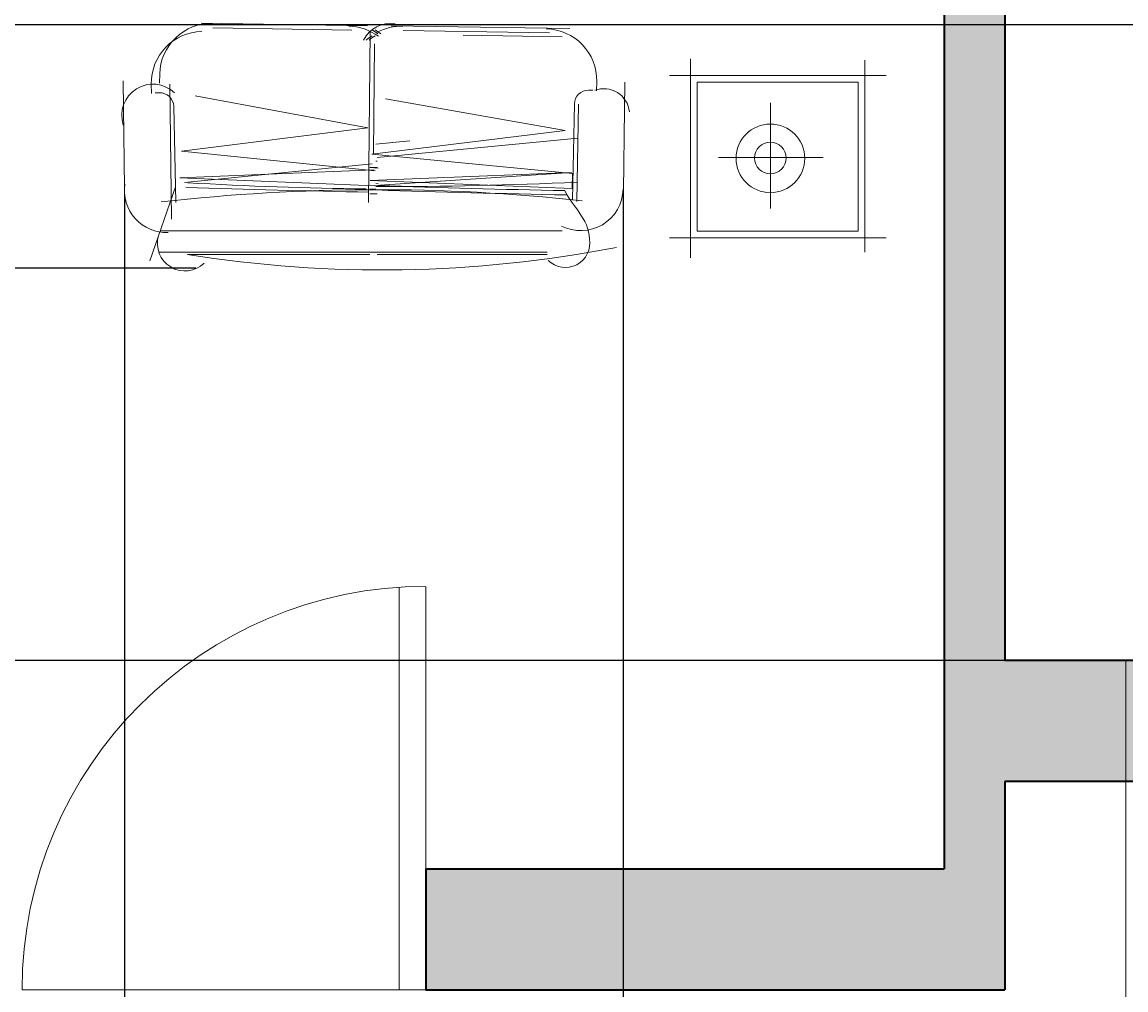
# Model space of a CAD drawing. Units: inches. Extents: x 2807 to 3326, y 2005 to 2580.
# Tile 4 of 12: x 3067 to 3149, y 2120 to 2192. Entities that reach past the tile are written whole.
import ezdxf

# ---------------------------------------------------------------- set-up
doc = ezdxf.new("R2010")
doc.units = ezdxf.units.IN
doc.header["$LTSCALE"] = 0.4
for name, color, linetype, lineweight in [('A-ANNO-DIMS', 2, 'Continuous', 18), ('A-FLOR-STRS', 233, 'Continuous', 18), ('A-WALL-PATT', 231, 'Continuous', 13), ('DOORS', 144, 'Continuous', 18), ('Furniture', 7, 'Continuous', 15), ('WALL', 233, 'Continuous', 35)]:
    doc.layers.add(name, color=color, linetype=linetype, lineweight=lineweight)
doc.styles.get("Standard").update_dxf_attribs({"font": 'txt', "height": 5})
doc.dimstyles.get("Standard").update_dxf_attribs({"dimtxt": 0.18, "dimasz": 0.18, "dimexe": 0.18, "dimexo": 0.0625, "dimgap": 0.09, "dimtad": 0, "dimtih": 1, "dimtoh": 1, "dimdec": 4, "dimzin": 0, "dimdsep": 46, "dimtxsty": 'Standard', "dimcen": 0.09, "dimadec": 0, "dimazin": 0, "dimtfac": 1, "dimtdec": 4, "dimtofl": 0, "dimtmove": 0, "dimatfit": 3, "dimfxl": 1, "dimtolj": 1, "dimtzin": 0, "dimarcsym": 0})

# ---------------------------------------------------------------- blocks, each defined once
blk = doc.blocks.new('DOOR-30')
for p, q in [((0, 0), (-30, 0)), ((-2, -29.933), (-2, 0)), ((0, -30), (0, 0))]:
    blk.add_line(p, q)
blk.add_arc((0, 0), 30, 180, 270)
blk = doc.blocks.new('*D31')
at = {"layer": 'A-ANNO-DIMS', "color": 0, "lineweight": -2, "ltscale": 0.4, "transparency": 16777216}
for p, q in [((2844.567, 2135.514), (2844.567, 2008.446)), ((3288.567, 2135.514), (3288.567, 2008.446)), ((2844.747, 2008.626), (3059.93, 2008.626)), ((3288.387, 2008.626), (3073.205, 2008.626))]:
    blk.add_line(p, q, dxfattribs=at)
at = {"layer": 'A-ANNO-DIMS', "color": 0, "ltscale": 0.4, "transparency": 16777216}
for points in [[(2844.747, 2008.656), (2844.747, 2008.596), (2844.567, 2008.626)], [(3288.387, 2008.656), (3288.387, 2008.596), (3288.567, 2008.626)]]:
    blk.add_solid(points, dxfattribs=at)
at = {"layer": 'Defpoints', "color": 0, "ltscale": 0.4, "transparency": 16777216}
for p in [(2844.567, 2135.576), (3288.567, 2135.576), (3288.567, 2008.626)]:
    blk.add_point(p, dxfattribs=at)
at = {"layer": 'A-ANNO-DIMS', "color": 0, "ltscale": 0.4, "transparency": 16777216, "insert": (3066.567, 2008.626), "char_height": 5, "attachment_point": 5}
blk.add_mtext('\\A1;444', dxfattribs=at)
blk = doc.blocks.new('*D45')
at = {"layer": 'A-ANNO-DIMS', "color": 0, "lineweight": -2, "ltscale": 0.4, "transparency": 16777216}
for p, q in [((3279.504691, 2191.826496), (2816.937191, 2191.826496)), ((2817.117191, 2191.646496), (2817.117191, 2170.791496)), ((2817.117191, 2144.756496), (2817.117191, 2165.611496)), ((3279.504691, 2144.576496), (2816.937191, 2144.576496))]:
    blk.add_line(p, q, dxfattribs=at)
at = {"layer": 'A-ANNO-DIMS', "color": 0, "ltscale": 0.4, "transparency": 16777216}
for points in [[(2817.087191, 2191.646496), (2817.147191, 2191.646496), (2817.117191, 2191.826496)], [(2817.087191, 2144.756496), (2817.147191, 2144.756496), (2817.117191, 2144.576496)]]:
    blk.add_solid(points, dxfattribs=at)
at = {"layer": 'Defpoints', "color": 0, "ltscale": 0.4, "transparency": 16777216}
for p in [(2817.117191, 2191.826496), (3279.567191, 2191.826496), (3279.567191, 2144.576496)]:
    blk.add_point(p, dxfattribs=at)
at = {"layer": 'A-ANNO-DIMS', "color": 0, "ltscale": 0.4, "transparency": 16777216, "insert": (2817.117191, 2168.201496), "char_height": 5, "attachment_point": 5}
blk.add_mtext('\\A1;47.25', dxfattribs=at)
blk = doc.blocks.new('*D61')
at = {"layer": 'A-ANNO-DIMS', "color": 0, "lineweight": -2, "ltscale": 0.4, "transparency": 16777216}
for p, q in [((3088.922898, 2267.452063), (2816.937191, 2267.452063)), ((2817.117191, 2267.272063), (2817.117191, 2223.175564)), ((2817.117191, 2173.899065), (2817.117191, 2217.995564)), ((3079.479513, 2173.719065), (2816.937191, 2173.719065))]:
    blk.add_line(p, q, dxfattribs=at)
at = {"layer": 'A-ANNO-DIMS', "color": 0, "ltscale": 0.4, "transparency": 16777216}
for points in [[(2817.087191, 2267.272063), (2817.147191, 2267.272063), (2817.117191, 2267.452063)], [(2817.087191, 2173.899065), (2817.147191, 2173.899065), (2817.117191, 2173.719065)]]:
    blk.add_solid(points, dxfattribs=at)
at = {"layer": 'Defpoints', "color": 0, "ltscale": 0.4, "transparency": 16777216}
for p in [(2817.117191, 2267.452063), (3088.985398, 2267.452063), (3079.542013, 2173.719065)]:
    blk.add_point(p, dxfattribs=at)
at = {"layer": 'A-ANNO-DIMS', "color": 0, "ltscale": 0.4, "transparency": 16777216, "insert": (2817.117191, 2220.585564), "char_height": 5, "attachment_point": 5}
blk.add_mtext('\\A1;93.73', dxfattribs=at)
blk = doc.blocks.new('*D62')
at = {"layer": 'A-ANNO-DIMS', "color": 0, "lineweight": -2, "ltscale": 0.4, "transparency": 16777216}
for p, q in [((3074.185, 2179.209), (3074.185, 2008.446)), ((3111.213, 2179.531), (3111.213, 2008.446)), ((3074.365, 2008.626), (3082.609, 2008.626)), ((3111.033, 2008.626), (3102.789, 2008.626))]:
    blk.add_line(p, q, dxfattribs=at)
at = {"layer": 'A-ANNO-DIMS', "color": 0, "ltscale": 0.4, "transparency": 16777216}
for points in [[(3074.365, 2008.656), (3074.365, 2008.596), (3074.185, 2008.626)], [(3111.033, 2008.656), (3111.033, 2008.596), (3111.213, 2008.626)]]:
    blk.add_solid(points, dxfattribs=at)
at = {"layer": 'Defpoints', "color": 0, "ltscale": 0.4, "transparency": 16777216}
for p in [(3111.213, 2179.594), (3074.185, 2179.271), (3111.213, 2008.626)]:
    blk.add_point(p, dxfattribs=at)
at = {"layer": 'A-ANNO-DIMS', "color": 0, "ltscale": 0.4, "transparency": 16777216, "insert": (3092.699, 2008.626), "char_height": 5, "attachment_point": 5}
blk.add_mtext('\\A1;37.03', dxfattribs=at)

msp = doc.modelspace()

# ---------------------------------------------------------------- hatches: boundary and pattern name
at = {"layer": 'A-WALL-PATT', "ltscale": 0.4}
h = msp.add_hatch(color=256, dxfattribs=at)
h.dxf.hatch_style = 1
h.paths.add_polyline_path([(3288.5672, 2549.5765), (2941.5672, 2549.5765), (2941.5672, 2540.5765), (2993.5672, 2540.5765), (2993.5672, 2489.5693), (2998.0672, 2489.5693), (2998.0672, 2540.5765), (3135.0672, 2540.5765), (3135.0672, 2479.0765), (3139.5672, 2479.0765), (3139.5672, 2540.5765), (3279.5672, 2540.5765), (3279.5672, 2510.5765), (3288.5672, 2510.5765)])
h.paths.add_polyline_path([(2905.5672, 2549.5765), (2844.5672, 2549.5765), (2844.5672, 2445.94), (2853.5672, 2445.94), (2853.5672, 2540.5765), (2905.5672, 2540.5765)])
h.paths.add_polyline_path([(2853.5672, 2409.94), (2844.5672, 2409.94), (2844.5672, 2371.3497), (2853.5672, 2371.3497), (2853.5672, 2380.0765), (2909.0672, 2380.0765), (2909.0672, 2384.5765), (2853.5672, 2384.5765)])
h.paths.add_polyline_path([(2998.0672, 2389.0765), (2993.5672, 2389.0765), (2993.5672, 2384.5765), (2939.0672, 2384.5765), (2939.0672, 2380.0765), (2943.5672, 2380.0765), (2943.5672, 2314.0765), (2948.0672, 2314.0765), (2948.0672, 2380.0765), (2998.0672, 2380.0765)])
h.paths.add_polyline_path([(2998.0672, 2471.8029), (2993.5672, 2471.8029), (2993.5672, 2425.0765), (2998.0672, 2425.0765)])
h.paths.add_polyline_path([(2953.0672, 2279.5765), (2948.0672, 2279.5765), (2948.0672, 2284.0765), (2943.5672, 2284.0765), (2943.5672, 2279.5765), (2853.5672, 2279.5765), (2853.5672, 2289.0663), (2844.5672, 2289.0663), (2844.5672, 2227.8961), (2853.5672, 2227.8961), (2853.5672, 2275.0765), (2953.0672, 2275.0765)])
h.paths.add_polyline_path([(2943.5672, 2332.0765), (2853.5672, 2332.0765), (2853.5672, 2347.3497), (2844.5672, 2347.3497), (2844.5672, 2313.0663), (2853.5672, 2313.0663), (2853.5672, 2327.5765), (2943.5672, 2327.5765)])
h.paths.add_polyline_path([(3144.0672, 2279.5765), (2993.5672, 2279.5765), (2989.0672, 2279.5765), (2989.0672, 2275.0765), (2993.5672, 2275.0765), (2993.5672, 2144.5765), (2984.5672, 2144.5765), (2984.5672, 2135.5765), (2993.5672, 2135.5765), (2993.5672, 2120.0765), (3036.5672, 2120.0765), (3036.5672, 2129.0765), (2998.0672, 2129.0765), (2998.0672, 2275.0765), (3135.0672, 2275.0765), (3135.0672, 2129.0765), (3096.5672, 2129.0765), (3096.5672, 2120.0765), (3139.5672, 2120.0765), (3139.5672, 2135.5765), (3148.5672, 2135.5765), (3148.5672, 2144.5765), (3139.5672, 2144.5765), (3139.5672, 2275.0765), (3144.0672, 2275.0765)])
h.paths.add_polyline_path([(2984.5672, 2144.5765), (2925.9914, 2144.5765), (2925.9914, 2135.5765), (2984.5672, 2135.5765)])
h.paths.add_polyline_path([(2889.9914, 2144.5765), (2853.5672, 2144.5765), (2853.5672, 2191.8961), (2844.5672, 2191.8961), (2844.5672, 2135.5765), (2889.9914, 2135.5765)])
h.paths.add_polyline_path([(3196.0672, 2144.5765), (3148.5672, 2144.5765), (3148.5672, 2135.5765), (3196.0672, 2135.5765)])
h.paths.add_polyline_path([(3288.5672, 2191.8265), (3279.5672, 2191.8265), (3279.5672, 2144.5765), (3232.0672, 2144.5765), (3232.0672, 2135.5765), (3288.5672, 2135.5765)])
h.paths.add_polyline_path([(3288.5672, 2292.8229), (3279.5672, 2292.8229), (3279.5672, 2291.4371), (3279.5672, 2279.5765), (3189.5672, 2279.5765), (3189.5672, 2293.0765), (3185.0672, 2293.0765), (3185.0672, 2279.5765), (3180.0672, 2279.5765), (3180.0672, 2275.0765), (3279.5672, 2275.0765), (3279.5672, 2227.8265), (3288.5672, 2227.8265)])
h.paths.add_polyline_path([(3288.5672, 2368.0765), (3279.5672, 2368.0765), (3279.5672, 2332.0765), (3174.0672, 2332.0765), (3174.0672, 2327.5765), (3185.0672, 2327.5765), (3189.5672, 2327.5765), (3279.5672, 2327.5765), (3279.5672, 2316.8229), (3288.5672, 2316.8229)])
h.paths.add_polyline_path([(3288.5672, 2474.5765), (3279.5672, 2474.5765), (3279.5672, 2444.5765), (3139.5672, 2444.5765), (3139.5672, 2449.0765), (3135.0672, 2449.0765), (3135.0672, 2327.5765), (3144.0672, 2327.5765), (3144.0672, 2332.0765), (3139.5672, 2332.0765), (3139.5672, 2440.0765), (3279.5672, 2440.0765), (3279.5672, 2404.0765), (3288.5672, 2404.0765)])

# ---------------------------------------------------------------- linework, layer by layer
at = {"layer": 'A-FLOR-STRS'}
msp.add_line((3148.5672, 2144.5765), (3148.5672, 2036.0765), dxfattribs=at)
at = {"layer": 'Furniture'}
for p, q in [((3092.2238, 2191.753), (3079.8624, 2191.9442)), ((3091.0734, 2191.4097), (3080.7301, 2191.5867)), ((3092.4259, 2191.3342), (3092.3073, 2178.6061)), ((3107.2561, 2191.5516), (3093.9972, 2191.7429)), ((3105.7383, 2191.2084), (3094.8649, 2191.3854)), ((3106.682, 2190.9339), (3099.3426, 2191.0504)), ((3092.7429, 2190.3922), (3092.6699, 2182.2476)), ((3116.2234, 2189.2884), (3116.2234, 2174.4943)), ((3129.174, 2174.9294), (3129.174, 2189.1796)), ((3076.7825, 2187.4841), (3076.7966, 2188.1681)), ((3076.7825, 2187.4841), (3076.7966, 2188.1681)), ((3130.7669, 2188.0407), (3114.6559, 2188.0407)), ((3074.2114, 2177.637), (3074.0852, 2187.6441)), ((3076.183, 2186.7231), (3076.1688, 2187.4072)), ((3077.5349, 2187.4066), (3077.6587, 2177.3736)), ((3108.6439, 2186.9564), (3108.9763, 2186.9496)), ((3109.2414, 2186.9145), (3109.2555, 2187.5985)), ((3111.3391, 2187.5603), (3111.2129, 2177.4345)), ((3116.7132, 2187.551), (3116.7132, 2176.4756)), ((3128.6842, 2187.551), (3116.7132, 2187.551)), ((3128.6842, 2176.4756), (3128.6842, 2187.551)), ((3076.7804, 2186.7651), (3076.4481, 2186.7582)), ((3092.2425, 2184.1562), (3079.4365, 2186.5282)), ((3106.9074, 2183.9549), (3093.5713, 2186.3269)), ((3077.8299, 2185.7581), (3077.9779, 2178.6061)), ((3107.5944, 2185.9495), (3107.4464, 2178.7974)), ((3107.8894, 2185.9187), (3107.7657, 2178.6873)), ((3122.1562, 2178.1736), (3122.1562, 2186.0117)), ((3078.4176, 2182.4123), (3092.2425, 2184.1562)), ((3092.5524, 2182.2109), (3106.9074, 2183.9549)), ((3092.8422, 2182.941), (3095.3643, 2183.1941)), ((3092.9551, 2181.9445), (3107.8461, 2183.3854)), ((3092.7914, 2180.9607), (3078.4176, 2182.4123)), ((3107.4562, 2180.7593), (3092.5524, 2182.2109)), ((3078.6364, 2180.0835), (3092.5706, 2181.4816)), ((3092.945, 2181.2396), (3092.3949, 2181.2161)), ((3093.0297, 2181.152), (3092.3949, 2181.2161)), ((3092.8422, 2181.6762), (3092.9551, 2181.6876)), ((3118.3079, 2181.9574), (3126.0886, 2181.9574)), ((3092.7066, 2181.0482), (3078.2975, 2180.4337)), ((3078.2975, 2180.4337), (3092.7722, 2179.8415)), ((3107.3715, 2180.8469), (3092.4323, 2180.2324)), ((3092.7712, 2179.8821), (3107.3715, 2180.8469)), ((3107.4371, 2179.6402), (3107.4562, 2180.7593)), ((3076.055, 2174.2607), (3077.9644, 2179.7681)), ((3092.4323, 2180.2324), (3107.4371, 2179.6402)), ((3092.8422, 2180.0398), (3093.0105, 2180.0329)), ((3092.4059, 2179.2603), (3092.8422, 2179.2603)), ((3092.8422, 2179.2603), (3092.9551, 2179.2603)), ((3076.8333, 2176.5055), (3092.4059, 2176.5055)), ((3092.4059, 2176.5055), (3092.8422, 2176.5055)), ((3092.8422, 2176.5055), (3092.9551, 2176.5055)), ((3092.9551, 2176.5055), (3106.697, 2176.5055)), ((3116.7132, 2176.4756), (3128.6842, 2176.4756)), ((3114.6559, 2175.9858), (3130.7669, 2175.9858)), ((3076.7268, 2174.9231), (3092.4059, 2174.9231)), ((3078.8971, 2174.7472), (3092.4059, 2174.7472)), ((3092.4059, 2174.9231), (3092.8422, 2174.9231)), ((3092.8422, 2174.9231), (3092.9551, 2174.9231)), ((3092.9551, 2174.9231), (3105.57, 2174.9231)), ((3092.9551, 2174.7472), (3105.57, 2174.7472))]:
    msp.add_line(p, q, dxfattribs=at)
for centre, radius in [((3122.1562, 2181.8902), 2.5525), ((3122.1562, 2181.9238), 1.1755)]:
    msp.add_circle(centre, radius, dxfattribs=at)
for centre, radius, start, end in [((3080.6345, 2188.0887), 3.8387, 88.814487, 178.814487), ((3093.9471, 2189.6664), 2.2574, 81.240011, 153.304404), ((3080.0067, 2187.4866), 3.8387, 91.185513, 181.185513), ((3090.7528, 2187.8793), 3.8387, 53.486293, 88.814487), ((3090.7195, 2188.0706), 3.8387, 53.486293, 61.168991), ((3090.9333, 2188.0706), 3.8387, 53.486293, 61.168991), ((3094.7693, 2187.8873), 3.8387, 88.814487, 118.203806), ((3105.4176, 2187.678), 3.8387, 358.814487, 88.814487), ((3094.5192, 2187.678), 3.8387, 120.50473, 128.408271), ((3094.7331, 2187.678), 3.8387, 120.50473, 128.408271), ((3076.2877, 2185.0877), 2.3178, 46.00951, 198.153774), ((3108.6227, 2185.9282), 1.0285, 88.814487, 178.814487), ((3109.7884, 2185.165), 1.9033, 5.650869, 110.597543), ((3076.8017, 2185.7368), 1.0285, 1.185513, 91.185513), ((3077.3024, 2179.4959), 3.1255, 171.465976, 272.136694), ((3092.9501, 2038.5942), 140.9674, 83.800923, 96.532861), ((3111.3353, 3135.0351), 955.851, 268.0457337, 268.8608168), ((3095.6005, 2472.7768), 293.179, 266.730785, 269.322598), ((3093.3113, 2472.7768), 293.179, 269.823059, 269.908321), ((3095.8388, 2472.9681), 293.179, 269.414373, 269.436435), ((3093.2901, 2495.0825), 315.2935, 269.939131, 272.635927), ((3118.5331, 2861.9887), 682.5923, 267.857629, 269.0216363), ((3108.0697, 2179.6589), 3.1439, 242.872897, 358.814487), ((3126.7405, 3210.7802), 1031.7974, 268.1190452, 268.9035573), ((3078.6659, 2175.5642), 2.0424, 163.262733, 314.552919), ((3106.9219, 2175.5966), 1.82, 225.425312, 10.014093), ((3093.3143, 2264.5772), 90.983, 260.83746, 281.034289)]:
    msp.add_arc(centre, radius, start, end, dxfattribs=at)
msp.add_open_spline([(3108.7143, 2175.9131), (3108.7382, 2177.3125), (3107.2064, 2178.6399), (3106.878, 2179.4959)], degree=3, dxfattribs=at)
at = {"layer": 'WALL'}
for p, q in [((3135.0672, 2275.0765), (3135.0672, 2129.0765)), ((3139.5672, 2275.0765), (3139.5672, 2144.5765)), ((3279.5672, 2144.5765), (3139.5672, 2144.5765)), ((3288.5672, 2135.5765), (3139.5672, 2135.5765)), ((3139.5672, 2135.5765), (3139.5672, 2120.0765)), ((3096.5672, 2129.0765), (3096.5672, 2120.0765)), ((3096.5672, 2129.0765), (3135.0672, 2129.0765)), ((3096.5672, 2120.0765), (3139.5672, 2120.0765))]:
    msp.add_line(p, q, dxfattribs=at)

# ---------------------------------------------------------------- block references
at = {"layer": 'DOORS', "extrusion": (0, 0, -1), "zscale": -1, "rotation": 180}
msp.add_blockref('DOOR-30', (-3096.5672, 2120.0765), dxfattribs=at)

# ---------------------------------------------------------------- dimensions: what is measured, and where the dimension line sits
at = {"layer": 'A-ANNO-DIMS', "ltscale": 0.4}
for base, p1, p2, picture, middle in [((2817.1172, 2267.4521), (3079.542, 2173.7191), (3088.9854, 2267.4521), '*D61', (2817.1172, 2220.5856)), ((2817.1172, 2191.8265), (3279.5672, 2144.5765), (3279.5672, 2191.8265), '*D45', (2817.1172, 2168.2015))]:
    dim = msp.add_linear_dim(base=base, p1=p1, p2=p2, angle=90, dimstyle='Standard', override={"dimdec": 2, "dimlfac": 1, "dimrnd": 0, "dimzin": 0, "dimdsep": 46, "dimlunit": 2}, dxfattribs=at)
    dim.commit()
    dim.dimension.update_dxf_attribs({"geometry": picture, "text_midpoint": middle})
for base, p1, p2, override, picture, middle in [((3111.2129, 2008.6265), (3074.1849, 2179.2711), (3111.2129, 2179.5939), {"dimdec": 2, "dimlfac": 1, "dimrnd": 0, "dimzin": 0, "dimdsep": 46, "dimlunit": 2}, '*D62', (3092.6989, 2008.6265)), ((3288.5672, 2008.6265), (2844.5672, 2135.5765), (3288.5672, 2135.5765), {"dimdec": 0, "dimlfac": 1, "dimrnd": 0, "dimzin": 0, "dimdsep": 46, "dimlunit": 2}, '*D31', (3066.5672, 2008.6265))]:
    dim = msp.add_linear_dim(base=base, p1=p1, p2=p2, dimstyle='Standard', override=override, dxfattribs=at)
    dim.commit()
    dim.dimension.update_dxf_attribs({"geometry": picture, "text_midpoint": middle})

doc.saveas('drawing.dxf')
